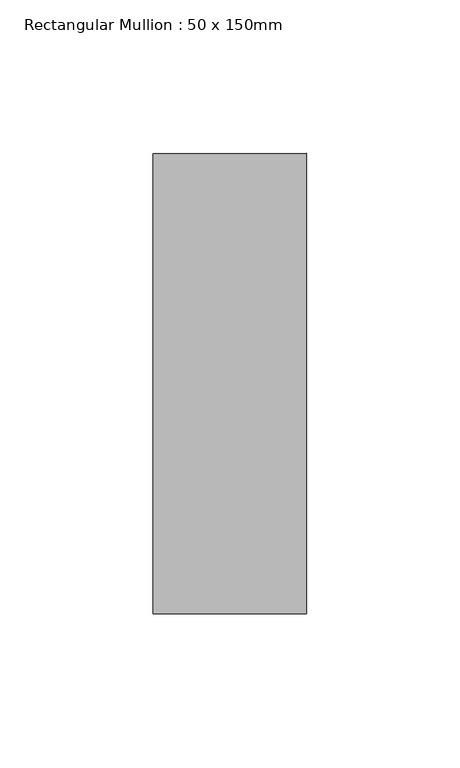
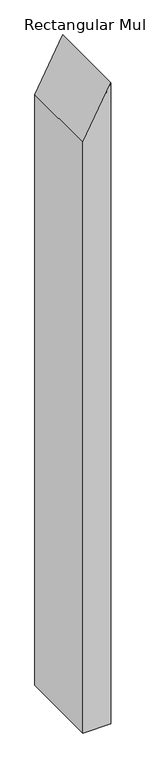
"""IFC4 building model written with IfcOpenShell, lengths in millimetres: member geometry, Rectangular Mullion : 50 x 150mm."""

from ifc_helpers import new_model, si_unit, frame, origin, place, context, project, spatial, polyline, outline, extrude, source, transform, mapped, element, save


def rectangular_mullion_50_x_150mm_6c5cdad2(model_context):
    return source(origin(), model_context, "Body", "SweptSolid", [
        extrude(outline(polyline([(0.0, 0.0), (-96.0491063, -50.0), (-1220.7745888, -50.0), (-1220.7745888, 0.0), (0.0, 0.0)])), frame((0.0, -75.0, 0.0), z_axis=(0.0, 1.0, 0.0), x_axis=(0.0, 0.0, 1.0)), (0.0, 0.0, 1.0), 150.0),
    ])


if __name__ == "__main__":
    model = new_model("IFC4")
    model_context = context("Model", 3, world=origin())
    ifc_project = project(units=[si_unit("LENGTHUNIT", "METRE", prefix="MILLI")], contexts=[model_context])
    site = spatial("IfcSite", under=ifc_project)
    building = spatial("IfcBuilding", under=site)
    placement = place(None, origin())
    rectangular_mullion_50_x_150mm_shape = rectangular_mullion_50_x_150mm_6c5cdad2(model_context)
    element("IfcMember", 1, ObjectType="Rectangular Mullion : 50 x 150mm", at=placement, inside=building, context=model_context, shape_type="MappedRepresentation", body=[
        mapped(rectangular_mullion_50_x_150mm_shape, transform((0.0, 0.0, 0.0), x_axis=(1.0, 0.0, 0.0), y_axis=(0.0, 1.0, 0.0), z_axis=(0.0, 0.0, 1.0))),
    ])
    save(model, "model.ifc")

# Revit data of these elements
# Type "Rectangular Mullion : 50 x 150mm"
#   built-in parameter 1007304 = 0.492126 (stored number, unit not read)
#   built-in parameter 1007301 = 0.082021 (stored number, unit not read)
#   built-in parameter 1007300 = 0.082021 (stored number, unit not read)
# Element 1 (IfcMember, "Rectangular Mullion : 50 x 150mm")
#   Materials on its faces: "Aluminium"
# Materials
#   "Aluminium": class "Metal", colour RGB 247 247 247, transparency 0, Description = "Aluminium 6061", Cost = 0
